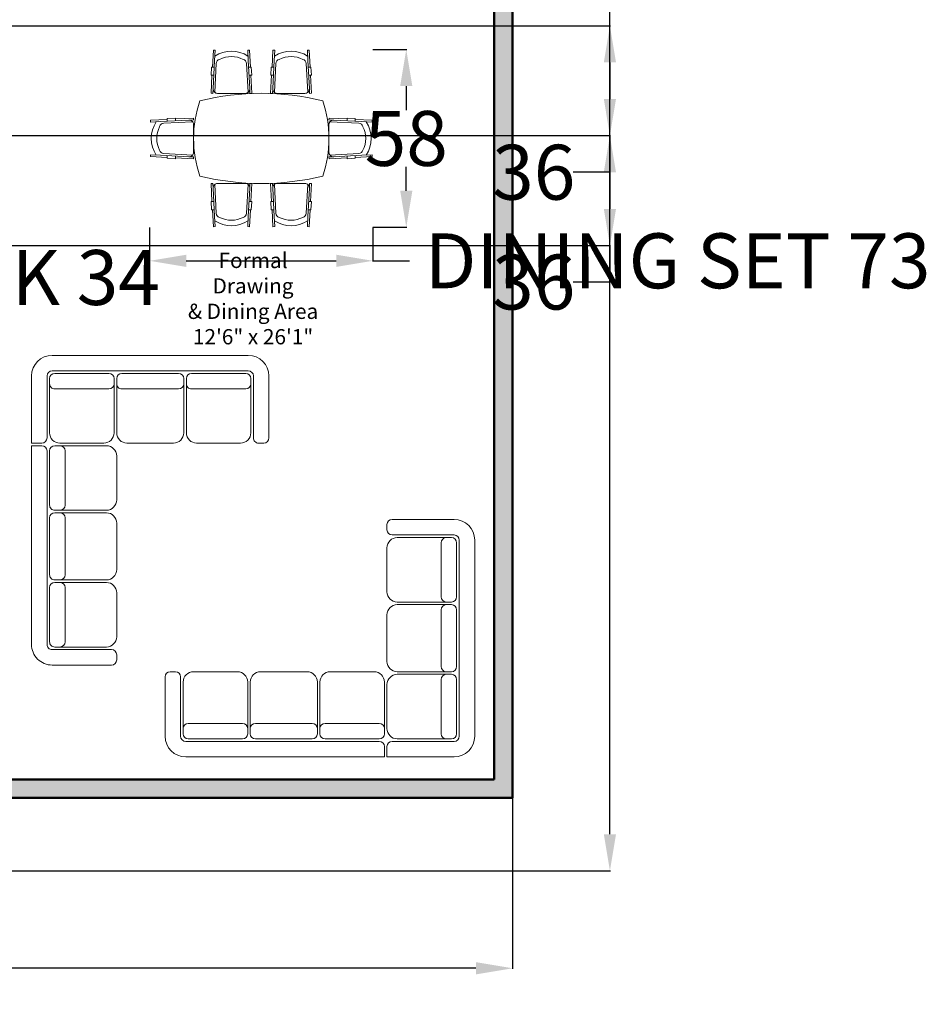
# Model space of a CAD drawing. Units: inches. Extents: x 2 to 695, y -374 to 352.
# Tile 2 of 6: x 398 to 695, y -374 to -51. Entities that reach past the tile are written whole.
import ezdxf

# ---------------------------------------------------------------- set-up
doc = ezdxf.new("R2010")
doc.units = ezdxf.units.IN
for name, color, linetype, lineweight in [('A-ANNO-DIMS', 2, 'Continuous', 18), ('A-AREA-IDEN', 7, 'Continuous', 18), ('A-WALL-PATT', 252, 'Continuous', 13), ('Furniture', 2, 'Continuous', 18), ('Outer Wall', 1, 'Continuous', 50)]:
    doc.layers.add(name, color=color, linetype=linetype, lineweight=lineweight)
doc.styles.get("Standard").update_dxf_attribs({"font": 'arial.ttf'})
doc.dimstyles.get("Standard").update_dxf_attribs({"dimtxt": 18, "dimasz": 12, "dimexe": 0.18, "dimexo": 0.0625, "dimgap": 0.09, "dimtad": 0, "dimtih": 1, "dimtoh": 1, "dimdec": 0, "dimzin": 0, "dimdsep": 46, "dimlunit": 3, "dimtxsty": 'Standard', "dimcen": 0.09, "dimadec": 0, "dimazin": 0, "dimtfac": 1, "dimtdec": 0, "dimtofl": 0, "dimtmove": 0, "dimatfit": 3, "dimfxl": 1, "dimtolj": 1, "dimtzin": 0, "dimarcsym": 0})

# ---------------------------------------------------------------- blocks, each defined once
blk = doc.blocks.new('A$C6BEF12A9')
for p, q in [((0.698, 1.955), (0.688, 1.768)), ((0.698, 1.955), (0.718, 1.954)), ((0.718, 1.954), (0.712, 1.841)), ((1.099, 1.955), (1.079, 1.954)), ((1.079, 1.954), (1.085, 1.841)), ((1.099, 1.955), (1.109, 1.768)), ((1.358, 1.955), (1.349, 1.768)), ((1.358, 1.955), (1.378, 1.954)), ((1.378, 1.954), (1.372, 1.841)), ((1.76, 1.955), (1.74, 1.954)), ((1.74, 1.954), (1.746, 1.841)), ((1.76, 1.955), (1.77, 1.768)), ((0.678, 1.768), (0.673, 1.678)), ((0.708, 1.768), (0.678, 1.768)), ((0.712, 1.841), (0.695, 1.529)), ((0.712, 1.841), (0.695, 1.529)), ((0.73, 1.806), (0.713, 1.488)), ((1.067, 1.806), (1.084, 1.488)), ((1.085, 1.841), (1.102, 1.529)), ((1.089, 1.768), (1.119, 1.768)), ((1.119, 1.768), (1.124, 1.678)), ((1.339, 1.768), (1.334, 1.678)), ((1.369, 1.768), (1.339, 1.768)), ((1.372, 1.841), (1.356, 1.529)), ((1.372, 1.841), (1.356, 1.529)), ((1.391, 1.806), (1.374, 1.488)), ((1.728, 1.806), (1.744, 1.488)), ((1.746, 1.841), (1.762, 1.529)), ((1.75, 1.768), (1.78, 1.768)), ((1.78, 1.768), (1.784, 1.678)), ((0.683, 1.678), (0.673, 1.477)), ((0.703, 1.678), (0.673, 1.678)), ((1.094, 1.678), (1.124, 1.678)), ((1.114, 1.678), (1.124, 1.477)), ((1.344, 1.678), (1.333, 1.477)), ((1.364, 1.678), (1.334, 1.678)), ((1.754, 1.678), (1.784, 1.678)), ((1.774, 1.678), (1.785, 1.477)), ((0.673, 1.477), (0.693, 1.476)), ((0.693, 1.476), (0.695, 1.526)), ((0.745, 1.476), (1.052, 1.476)), ((1.104, 1.476), (1.102, 1.526)), ((1.124, 1.477), (1.104, 1.476)), ((1.333, 1.477), (1.353, 1.476)), ((1.353, 1.476), (1.356, 1.526)), ((1.406, 1.476), (1.712, 1.476)), ((1.765, 1.476), (1.762, 1.526)), ((1.785, 1.477), (1.765, 1.476)), ((0.187, 1.198), (0.277, 1.203)), ((0.277, 1.193), (0.477, 1.203)), ((0.277, 1.173), (0.277, 1.203)), ((0.477, 1.203), (0.479, 1.183)), ((1.98, 1.203), (1.979, 1.183)), ((2.18, 1.193), (1.98, 1.203)), ((2.18, 1.173), (2.18, 1.203)), ((2.27, 1.198), (2.18, 1.203)), ((0, 1.178), (0.187, 1.188)), ((0, 1.178), (0.001, 1.158)), ((0.001, 1.158), (0.114, 1.164)), ((0.114, 1.164), (0.426, 1.181)), ((0.149, 1.146), (0.467, 1.163)), ((0.187, 1.168), (0.187, 1.198)), ((0.479, 1.183), (0.429, 1.181)), ((0.479, 0.824), (0.479, 1.131)), ((1.979, 1.183), (2.029, 1.181)), ((1.979, 0.824), (1.979, 1.131)), ((2.309, 1.146), (1.99, 1.163)), ((2.343, 1.164), (2.031, 1.181)), ((2.27, 1.168), (2.27, 1.198)), ((2.458, 1.178), (2.27, 1.188)), ((2.457, 1.158), (2.343, 1.164)), ((2.458, 1.178), (2.457, 1.158)), ((0, 0.777), (0.001, 0.797)), ((0, 0.777), (0.187, 0.767)), ((0.001, 0.797), (0.114, 0.791)), ((0.114, 0.791), (0.426, 0.774)), ((0.114, 0.791), (0.426, 0.774)), ((0.149, 0.809), (0.467, 0.792)), ((0.187, 0.787), (0.187, 0.757)), ((0.277, 0.782), (0.277, 0.752)), ((0.479, 0.772), (0.429, 0.774)), ((0.477, 0.752), (0.479, 0.772)), ((1.979, 0.772), (2.029, 0.774)), ((1.98, 0.752), (1.979, 0.772)), ((2.309, 0.809), (1.99, 0.792)), ((2.343, 0.791), (2.031, 0.774)), ((2.343, 0.791), (2.031, 0.774)), ((2.18, 0.782), (2.18, 0.752)), ((2.27, 0.787), (2.27, 0.757)), ((2.458, 0.777), (2.27, 0.767)), ((2.457, 0.797), (2.343, 0.791)), ((2.458, 0.777), (2.457, 0.797)), ((0.187, 0.757), (0.277, 0.752)), ((0.277, 0.762), (0.477, 0.752)), ((2.18, 0.762), (1.98, 0.752)), ((2.27, 0.757), (2.18, 0.752)), ((0.673, 0.477), (0.693, 0.479)), ((0.683, 0.277), (0.673, 0.477)), ((0.693, 0.479), (0.695, 0.429)), ((0.73, 0.149), (0.713, 0.467)), ((0.745, 0.479), (1.052, 0.479)), ((1.067, 0.149), (1.084, 0.467)), ((1.104, 0.479), (1.102, 0.429)), ((1.124, 0.477), (1.104, 0.479)), ((1.114, 0.277), (1.124, 0.477)), ((1.333, 0.477), (1.353, 0.479)), ((1.344, 0.277), (1.333, 0.477)), ((1.353, 0.479), (1.356, 0.429)), ((1.391, 0.149), (1.374, 0.467)), ((1.406, 0.479), (1.712, 0.479)), ((1.728, 0.149), (1.744, 0.467)), ((1.765, 0.479), (1.762, 0.429)), ((1.785, 0.477), (1.765, 0.479)), ((1.774, 0.277), (1.785, 0.477)), ((0.712, 0.114), (0.695, 0.426)), ((0.712, 0.114), (0.695, 0.426)), ((1.085, 0.114), (1.102, 0.426)), ((1.372, 0.114), (1.356, 0.426)), ((1.372, 0.114), (1.356, 0.426)), ((1.746, 0.114), (1.762, 0.426)), ((0.678, 0.187), (0.673, 0.277)), ((0.703, 0.277), (0.673, 0.277)), ((1.094, 0.277), (1.124, 0.277)), ((1.119, 0.187), (1.124, 0.277)), ((1.364, 0.277), (1.334, 0.277)), ((1.339, 0.187), (1.334, 0.277)), ((1.754, 0.277), (1.784, 0.277)), ((1.78, 0.187), (1.784, 0.277)), ((0.708, 0.187), (0.678, 0.187)), ((0.698, 0), (0.688, 0.187)), ((0.718, 0.001), (0.712, 0.114)), ((1.079, 0.001), (1.085, 0.114)), ((1.089, 0.187), (1.119, 0.187)), ((1.099, 0), (1.109, 0.187)), ((1.369, 0.187), (1.339, 0.187)), ((1.358, 0), (1.349, 0.187)), ((1.378, 0.001), (1.372, 0.114)), ((1.74, 0.001), (1.746, 0.114)), ((1.75, 0.187), (1.78, 0.187)), ((1.76, 0), (1.77, 0.187)), ((0.698, 0), (0.718, 0.001)), ((1.099, 0), (1.079, 0.001)), ((1.358, 0), (1.378, 0.001)), ((1.76, 0), (1.74, 0.001))]:
    blk.add_line(p, q)
for centre, radius, start, end in [((0.898, 1.603), 0.341, 57.3412, 122.6588), ((0.898, 1.603), 0.281, 62.3651, 117.6349), ((1.559, 1.603), 0.341, 57.3412, 122.6588), ((1.559, 1.603), 0.281, 62.3651, 117.6349), ((0.78, 1.804), 0.05, 103.7138, 177), ((1.017, 1.804), 0.05, 3, 76.2862), ((1.441, 1.804), 0.05, 103.7138, 177), ((1.678, 1.804), 0.05, 3, 76.2862), ((0.745, 1.526), 0.05, 177, 270), ((1.052, 1.526), 0.05, 270, 3), ((1.406, 1.526), 0.05, 177, 270), ((1.712, 1.526), 0.05, 270, 3), ((1.229, -1.385), 2.862, 76.2365, 103.7635), ((1.779, 0.977), 1.3, 161.253, 198.747), ((0.679, 0.977), 1.3, 341.253, 18.747), ((0.352, 0.977), 0.341, 147.3412, 212.6588), ((0.352, 0.977), 0.281, 152.3651, 207.6349), ((0.151, 1.096), 0.05, 93, 166.2862), ((0.429, 1.131), 0.05, 0, 93), ((2.029, 1.131), 0.05, 87, 180), ((2.306, 1.096), 0.05, 13.7138, 87), ((2.106, 0.977), 0.281, 332.3651, 27.6349), ((2.106, 0.977), 0.341, 327.3412, 32.6588), ((0.151, 0.859), 0.05, 193.7138, 267), ((0.429, 0.824), 0.05, 267, 0), ((2.029, 0.824), 0.05, 180, 273), ((2.306, 0.859), 0.05, 273, 346.2862), ((1.229, 3.34), 2.862, 256.2365, 283.7635), ((0.745, 0.429), 0.05, 90, 183), ((1.052, 0.429), 0.05, 357, 90), ((1.406, 0.429), 0.05, 90, 183), ((1.712, 0.429), 0.05, 357, 90), ((0.78, 0.151), 0.05, 183, 256.2862), ((1.017, 0.151), 0.05, 283.7138, 357), ((1.441, 0.151), 0.05, 183, 256.2862), ((1.678, 0.151), 0.05, 283.7138, 357), ((0.898, 0.352), 0.341, 237.3412, 302.6588), ((0.898, 0.352), 0.281, 242.3651, 297.6349), ((1.559, 0.352), 0.341, 237.3412, 302.6588), ((1.559, 0.352), 0.281, 242.3651, 297.6349)]:
    blk.add_arc(centre, radius, start, end)
blk = doc.blocks.new('A$C2AFA021D')
for p, q in [((0.8, 2.3), (0.2, 2.3)), ((0.85, 2.2), (0.85, 2.25)), ((0, 2.1), (0, 0.2)), ((0.15, 0.2), (0.15, 2.1)), ((0.2, 2.15), (0.8, 2.15)), ((0.225, 2.125), (0.275, 2.125)), ((0.75, 2.125), (0.275, 2.125)), ((0.175, 1.55), (0.175, 2.075)), ((0.325, 2.075), (0.325, 1.55)), ((0.85, 1.6), (0.85, 2.025)), ((0.275, 1.5), (0.225, 1.5)), ((0.225, 1.475), (0.275, 1.475)), ((0.275, 1.5), (0.75, 1.5)), ((0.75, 1.475), (0.275, 1.475)), ((0.175, 0.875), (0.175, 1.425)), ((0.325, 1.425), (0.325, 0.875)), ((0.85, 0.925), (0.85, 1.375)), ((0.275, 0.825), (0.225, 0.825)), ((0.225, 0.8), (0.275, 0.8)), ((0.275, 0.825), (0.75, 0.825)), ((0.75, 0.8), (0.275, 0.8)), ((0.975, 0.825), (1.4, 0.825)), ((1.625, 0.825), (2.075, 0.825)), ((2.3, 0.825), (2.725, 0.825)), ((2.85, 0.2), (2.85, 0.775)), ((2.9, 0.825), (2.95, 0.825)), ((3, 0.775), (3, 0.2)), ((0.175, 0.225), (0.175, 0.75)), ((0.325, 0.75), (0.325, 0.225)), ((0.85, 0.275), (0.85, 0.7)), ((0.875, 0.275), (0.875, 0.725)), ((1.5, 0.725), (1.5, 0.275)), ((1.525, 0.275), (1.525, 0.725)), ((2.175, 0.725), (2.175, 0.275)), ((2.2, 0.275), (2.2, 0.725)), ((2.825, 0.725), (2.825, 0.275)), ((1.45, 0.325), (0.925, 0.325)), ((2.125, 0.325), (1.575, 0.325)), ((2.775, 0.325), (2.25, 0.325)), ((0.875, 0.275), (0.875, 0.225)), ((1.5, 0.225), (1.5, 0.275)), ((1.525, 0.275), (1.525, 0.225)), ((2.175, 0.225), (2.175, 0.275)), ((2.2, 0.275), (2.2, 0.225)), ((2.825, 0.225), (2.825, 0.275)), ((0.8, 0.15), (0.2, 0.15)), ((0.275, 0.175), (0.225, 0.175)), ((0.275, 0.175), (0.75, 0.175)), ((0.85, 0), (0.85, 0.1)), ((0.875, 0.1), (0.875, 0)), ((0.925, 0.175), (1.45, 0.175)), ((0.925, 0.15), (2.8, 0.15)), ((1.575, 0.175), (2.125, 0.175)), ((2.25, 0.175), (2.775, 0.175)), ((0.2, 0), (0.85, 0)), ((2.8, 0), (0.875, 0))]:
    blk.add_line(p, q)
for centre, radius, start, end in [((0.2, 2.1), 0.2, 90, 180), ((0.8, 2.25), 0.05, 0, 90), ((0.8, 2.2), 0.05, 270, 0), ((0.2, 2.1), 0.05, 90, 180), ((0.225, 2.075), 0.05, 90, 180), ((0.275, 2.075), 0.05, 0, 90), ((0.75, 2.025), 0.1, 0, 90), ((0.225, 1.55), 0.05, 180, 270), ((0.275, 1.55), 0.05, 270, 0), ((0.75, 1.6), 0.1, 270, 0), ((0.225, 1.425), 0.05, 90, 180), ((0.275, 1.425), 0.05, 0, 90), ((0.75, 1.375), 0.1, 360, 90), ((0.225, 0.875), 0.05, 180, 270), ((0.275, 0.875), 0.05, 270, 0), ((0.75, 0.925), 0.1, 270, 0), ((0.225, 0.75), 0.05, 90, 180), ((0.275, 0.75), 0.05, 0, 90), ((0.75, 0.7), 0.1, 0, 90), ((0.975, 0.725), 0.1, 90, 180), ((1.4, 0.725), 0.1, 0, 90), ((1.625, 0.725), 0.1, 90, 180), ((2.075, 0.725), 0.1, 0, 90), ((2.3, 0.725), 0.1, 90, 180), ((2.725, 0.725), 0.1, 0, 90), ((2.9, 0.775), 0.05, 90, 180), ((2.95, 0.775), 0.05, 0, 90), ((0.925, 0.275), 0.05, 90, 180), ((1.45, 0.275), 0.05, 360, 90), ((1.575, 0.275), 0.05, 90, 180), ((2.125, 0.275), 0.05, 360, 90), ((2.25, 0.275), 0.05, 90, 180), ((2.775, 0.275), 0.05, 360, 90), ((0.2, 0.2), 0.2, 180, 270), ((0.2, 0.2), 0.05, 180, 270), ((0.225, 0.225), 0.05, 180, 270), ((0.275, 0.225), 0.05, 270, 0), ((0.75, 0.275), 0.1, 270, 0), ((0.925, 0.225), 0.05, 180, 270), ((1.45, 0.225), 0.05, 270, 0), ((1.575, 0.225), 0.05, 180, 270), ((2.125, 0.225), 0.05, 270, 0), ((2.25, 0.225), 0.05, 180, 270), ((2.775, 0.225), 0.05, 270, 0), ((2.8, 0.2), 0.2, 270, 0), ((2.8, 0.2), 0.05, 270, 0), ((0.8, 0.1), 0.05, 0, 90), ((0.925, 0.1), 0.05, 90, 180)]:
    blk.add_arc(centre, radius, start, end)
blk = doc.blocks.new('*D20')
at = {"layer": 'A-ANNO-DIMS', "color": 0, "lineweight": -2, "transparency": 16777216}
for p, q in [((440.79, -118.95), (440.79, -130.04)), ((513.95, -118.95), (513.95, -130.04)), ((452.79, -129.86), (501.95, -129.86)), ((513.95, -129.86), (525.95, -129.86))]:
    blk.add_line(p, q, dxfattribs=at)
at = {"layer": 'A-ANNO-DIMS', "color": 0, "transparency": 16777216}
for points in [[(452.79, -127.86), (452.79, -131.86), (440.79, -129.86)], [(501.95, -127.86), (501.95, -131.86), (513.95, -129.86)]]:
    blk.add_solid(points, dxfattribs=at)
at = {"layer": 'Defpoints', "color": 0, "transparency": 16777216}
for p in [(440.79, -118.88), (513.95, -118.88), (513.95, -129.86)]:
    blk.add_point(p, dxfattribs=at)
at = {"layer": 'A-ANNO-DIMS', "color": 0, "transparency": 16777216, "insert": (613.93, -129.86), "char_height": 18, "attachment_point": 5}
blk.add_mtext('\\A1;DINING SET 73', dxfattribs=at)
blk = doc.blocks.new('*D21')
at = {"layer": 'A-ANNO-DIMS', "color": 0, "lineweight": -2, "transparency": 16777216}
for p, q in [((514.02, -60.6), (525.11, -60.6)), ((524.93, -72.6), (524.93, -80.46)), ((524.93, -106.88), (524.93, -99.02)), ((514.02, -118.88), (525.11, -118.88))]:
    blk.add_line(p, q, dxfattribs=at)
at = {"layer": 'A-ANNO-DIMS', "color": 0, "transparency": 16777216}
for points in [[(522.93, -72.6), (526.93, -72.6), (524.93, -60.6)], [(522.93, -106.88), (526.93, -106.88), (524.93, -118.88)]]:
    blk.add_solid(points, dxfattribs=at)
at = {"layer": 'Defpoints', "color": 0, "transparency": 16777216}
for p in [(513.95, -60.6), (524.93, -60.6), (513.95, -118.88)]:
    blk.add_point(p, dxfattribs=at)
at = {"layer": 'A-ANNO-DIMS', "color": 0, "transparency": 16777216, "insert": (524.93, -89.74), "char_height": 18, "attachment_point": 5}
blk.add_mtext('\\A1;58', dxfattribs=at)
blk = doc.blocks.new('*D22')
at = {"layer": 'A-ANNO-DIMS', "color": 0, "lineweight": -2, "transparency": 16777216}
for p, q in [((308.29, -140.37), (308.29, -135.15)), ((320.29, -135.33), (330.3, -135.33)), ((342.3, -140.37), (342.3, -135.15)), ((342.3, -135.33), (354.3, -135.33))]:
    blk.add_line(p, q, dxfattribs=at)
at = {"layer": 'A-ANNO-DIMS', "color": 0, "transparency": 16777216}
for points in [[(320.29, -133.33), (320.29, -137.33), (308.29, -135.33)], [(330.3, -133.33), (330.3, -137.33), (342.3, -135.33)]]:
    blk.add_solid(points, dxfattribs=at)
at = {"layer": 'Defpoints', "color": 0, "transparency": 16777216}
for p in [(342.3, -135.33), (308.29, -140.43), (342.3, -140.43)]:
    blk.add_point(p, dxfattribs=at)
at = {"layer": 'A-ANNO-DIMS', "color": 0, "transparency": 16777216, "insert": (400.04, -135.33), "char_height": 18, "attachment_point": 5}
blk.add_mtext('\\A1;SINK 34', dxfattribs=at)
blk = doc.blocks.new('*D28')
at = {"layer": 'A-ANNO-DIMS', "color": 0, "lineweight": -2, "transparency": 16777216}
for p, q in [((559.79, -305.89), (559.79, -361.92)), ((146.79, -329.89), (146.79, -361.92)), ((158.79, -361.74), (332.95, -361.74)), ((547.79, -361.74), (373.62, -361.74))]:
    blk.add_line(p, q, dxfattribs=at)
at = {"layer": 'A-ANNO-DIMS', "color": 0, "transparency": 16777216}
for points in [[(158.79, -359.74), (158.79, -363.74), (146.79, -361.74)], [(547.79, -359.74), (547.79, -363.74), (559.79, -361.74)]]:
    blk.add_solid(points, dxfattribs=at)
at = {"layer": 'Defpoints', "color": 0, "transparency": 16777216}
for p in [(559.79, -305.82), (146.79, -329.82), (559.79, -361.74)]:
    blk.add_point(p, dxfattribs=at)
at = {"layer": 'A-ANNO-DIMS', "color": 0, "transparency": 16777216, "insert": (353.29, -361.74), "char_height": 18, "attachment_point": 5}
blk.add_mtext('\\A1;413', dxfattribs=at)
blk = doc.blocks.new('*D29')
at = {"layer": 'A-ANNO-DIMS', "color": 0, "lineweight": -2, "transparency": 16777216}
for p, q in [((420.85, 308.13), (591.88, 308.13)), ((591.7, 296.13), (591.7, -1.56)), ((591.7, -317.82), (591.7, -20.13)), ((217.35, -329.82), (591.88, -329.82))]:
    blk.add_line(p, q, dxfattribs=at)
at = {"layer": 'A-ANNO-DIMS', "color": 0, "transparency": 16777216}
for points in [[(589.7, 296.13), (593.7, 296.13), (591.7, 308.13)], [(589.7, -317.82), (593.7, -317.82), (591.7, -329.82)]]:
    blk.add_solid(points, dxfattribs=at)
at = {"layer": 'Defpoints', "color": 0, "transparency": 16777216}
for p in [(420.79, 308.13), (591.7, 308.13), (217.29, -329.82)]:
    blk.add_point(p, dxfattribs=at)
at = {"layer": 'A-ANNO-DIMS', "color": 0, "transparency": 16777216, "insert": (591.7, -10.85), "char_height": 18, "attachment_point": 5}
blk.add_mtext('\\A1;638', dxfattribs=at)
blk = doc.blocks.new('*D37')
at = {"layer": 'A-ANNO-DIMS', "color": 0, "lineweight": -2, "transparency": 16777216}
for p, q in [((350.85, -88.82), (591.88, -88.82)), ((591.7, -100.82), (591.7, -112.82)), ((350.85, -124.82), (591.88, -124.82)), ((591.7, -124.82), (591.7, -136.82)), ((591.7, -136.82), (579.7, -136.82))]:
    blk.add_line(p, q, dxfattribs=at)
at = {"layer": 'A-ANNO-DIMS', "color": 0, "transparency": 16777216}
for points in [[(589.7, -100.82), (593.7, -100.82), (591.7, -88.82)], [(589.7, -112.82), (593.7, -112.82), (591.7, -124.82)]]:
    blk.add_solid(points, dxfattribs=at)
at = {"layer": 'Defpoints', "color": 0, "transparency": 16777216}
for p in [(350.79, -88.82), (350.79, -124.82), (591.7, -124.82)]:
    blk.add_point(p, dxfattribs=at)
at = {"layer": 'A-ANNO-DIMS', "color": 0, "transparency": 16777216, "insert": (566.73, -136.82), "char_height": 18, "attachment_point": 5}
blk.add_mtext('\\A1;36', dxfattribs=at)
blk = doc.blocks.new('*D41')
at = {"layer": 'A-ANNO-DIMS', "color": 0, "lineweight": -2, "transparency": 16777216}
for p, q in [((342.285845, 340.044756), (330.285845, 340.044756)), ((354.285845, -164.762454), (354.285845, 340.224756)), ((390.285845, -164.762454), (390.285845, 340.224756)), ((402.285845, 340.044756), (414.285845, 340.044756))]:
    blk.add_line(p, q, dxfattribs=at)
at = {"layer": 'A-ANNO-DIMS', "color": 0, "transparency": 16777216}
for points in [[(342.285845, 342.044756), (342.285845, 338.044756), (354.285845, 340.044756)], [(402.285845, 342.044756), (402.285845, 338.044756), (390.285845, 340.044756)]]:
    blk.add_solid(points, dxfattribs=at)
at = {"layer": 'Defpoints', "color": 0, "transparency": 16777216}
for p in [(390.285845, 340.044756), (354.285845, -164.824954), (390.285845, -164.824954)]:
    blk.add_point(p, dxfattribs=at)
at = {"layer": 'A-ANNO-DIMS', "color": 0, "transparency": 16777216, "insert": (372.285845, 340.044756), "char_height": 18, "attachment_point": 5}
blk.add_mtext('\\A1;36', dxfattribs=at)
blk = doc.blocks.new('*D51')
at = {"layer": 'A-ANNO-DIMS', "color": 0, "lineweight": -2, "transparency": 16777216}
for p, q in [((346.85, -52.82), (591.88, -52.82)), ((591.7, -64.82), (591.7, -76.82)), ((346.85, -88.82), (591.88, -88.82)), ((591.7, -88.82), (591.7, -100.82)), ((591.7, -100.82), (579.7, -100.82))]:
    blk.add_line(p, q, dxfattribs=at)
at = {"layer": 'A-ANNO-DIMS', "color": 0, "transparency": 16777216}
for points in [[(589.7, -64.82), (593.7, -64.82), (591.7, -52.82)], [(589.7, -76.82), (593.7, -76.82), (591.7, -88.82)]]:
    blk.add_solid(points, dxfattribs=at)
at = {"layer": 'Defpoints', "color": 0, "transparency": 16777216}
for p in [(346.79, -52.82), (346.79, -88.82), (591.7, -88.82)]:
    blk.add_point(p, dxfattribs=at)
at = {"layer": 'A-ANNO-DIMS', "color": 0, "transparency": 16777216, "insert": (566.73, -100.82), "char_height": 18, "attachment_point": 5}
blk.add_mtext('\\A1;36', dxfattribs=at)

msp = doc.modelspace()

# ---------------------------------------------------------------- hatches: boundary and pattern name
at = {"layer": 'A-WALL-PATT'}
h = msp.add_hatch(color=256, dxfattribs=at)
h.dxf.hatch_style = 1
h.paths.add_polyline_path([(346.7858, 296.175), (146.7858, 296.175), (146.7858, -329.825), (217.2858, -329.825), (217.2858, -305.825), (559.7858, -305.825), (559.7858, 296.175), (420.7858, 296.175), (420.7858, 290.175), (553.7858, 290.175), (553.7858, -299.825), (213.2858, -299.825), (213.2858, -323.825), (152.7858, -323.825), (152.7858, 290.175), (346.7858, 290.175)])
h.paths.add_polyline_path([(420.7858, 308.1298), (346.7858, 308.1298), (346.7858, 242.175), (228.7858, 242.175), (228.7858, 264.175), (152.7858, 264.175), (152.7858, 260.175), (224.7858, 260.175), (224.7858, 236.175), (350.7858, 236.175), (350.7858, 302.1298), (416.7858, 302.1298), (416.7858, 236.175), (553.7858, 236.175), (553.7858, 242.175), (420.7858, 242.175)])

# ---------------------------------------------------------------- linework, layer by layer
at = {"layer": 'Outer Wall'}
for p, q in [((559.7858, -305.825), (559.7858, 296.175)), ((553.7858, -299.825), (553.7858, 290.175)), ((553.7858, -299.825), (213.2858, -299.825)), ((559.7858, -305.825), (217.2858, -305.825))]:
    msp.add_line(p, q, dxfattribs=at)

# ---------------------------------------------------------------- block references
at = {"layer": 'Furniture'}
for name, p, xscale, yscale, zscale in [('A$C6BEF12A9', (441.0113, -118.6658), 29.59247402267948, 29.59247402267948, 29.59247402267948), ('A$C2AFA021D', (547.3739, -292.4654), -33.84012530478223, 33.84012530478223, 33.84012530478223)]:
    msp.add_blockref(name, p, dxfattribs=dict(at, xscale=xscale, yscale=yscale, zscale=zscale))
at = {"layer": 'Furniture', "xscale": 33.84012530478223, "yscale": 33.84012530478223, "zscale": 33.84012530478223, "rotation": 270}
msp.add_blockref('A$C2AFA021D', (402.0547, -160.8417), dxfattribs=at)

# ---------------------------------------------------------------- texts
at = {"layer": 'A-AREA-IDEN', "insert": (499.2436, -127.2325), "char_height": 5, "attachment_point": 3}
msp.add_mtext_dynamic_manual_height_columns('\\pxqc;{\\fTimes New Roman|b0|i0|c0|p18;Formal Drawing \\P& Dining Area\\P12\'6" x 26\'1"}', width=49.101878, gutter_width=12.5, heights=[0], dxfattribs=at)

# ---------------------------------------------------------------- dimensions: what is measured, and where the dimension line sits
at = {"layer": 'A-ANNO-DIMS'}
for base, p1, p2, picture, middle in [((390.2858, 340.0448), (354.2858, -164.825), (390.2858, -164.825), '*D41', (372.2858, 340.0448)), ((559.7858, -361.74), (146.7858, -329.825), (559.7858, -305.825), '*D28', (353.2858, -361.74))]:
    dim = msp.add_linear_dim(base=base, p1=p1, p2=p2, dimstyle='Standard', override={"dimdec": 0, "dimlfac": 1, "dimrnd": 0, "dimzin": 0, "dimdsep": 46, "dimlunit": 2}, dxfattribs=at)
    dim.commit()
    dim.dimension.update_dxf_attribs({"geometry": picture, "text_midpoint": middle})
for base, p1, p2, picture, middle in [((591.7008, 308.1298), (217.2858, -329.825), (420.7858, 308.1298), '*D29', (591.7008, -10.8476)), ((591.7008, -88.825), (346.7858, -52.825), (346.7858, -88.825), '*D51', (566.7309, -100.825)), ((524.9288, -60.5975), (513.9546, -118.8833), (513.9546, -60.5975), '*D21', (524.9288, -89.7404)), ((591.7008, -124.825), (350.7858, -88.825), (350.7858, -124.825), '*D37', (566.7309, -136.825))]:
    dim = msp.add_linear_dim(base=base, p1=p1, p2=p2, angle=90, dimstyle='Standard', override={"dimdec": 0, "dimlfac": 1, "dimrnd": 0, "dimzin": 0, "dimdsep": 46, "dimlunit": 2}, dxfattribs=at)
    dim.commit()
    dim.dimension.update_dxf_attribs({"geometry": picture, "text_midpoint": middle})
for base, p1, p2, text, picture, middle in [((513.9546, -129.8574), (440.7938, -118.8833), (513.9546, -118.8833), 'DINING SET <>', '*D20', (613.9328, -129.8574)), ((342.3028, -135.3283), (308.2945, -140.4295), (342.3028, -140.4295), 'SINK <>', '*D22', (400.0436, -135.3283))]:
    dim = msp.add_linear_dim(base=base, p1=p1, p2=p2, text=text, dimstyle='Standard', override={"dimdec": 0, "dimlfac": 1, "dimrnd": 0, "dimzin": 0, "dimdsep": 46, "dimlunit": 2}, dxfattribs=at)
    dim.commit()
    dim.dimension.update_dxf_attribs({"geometry": picture, "text_midpoint": middle})

doc.saveas('drawing.dxf')
